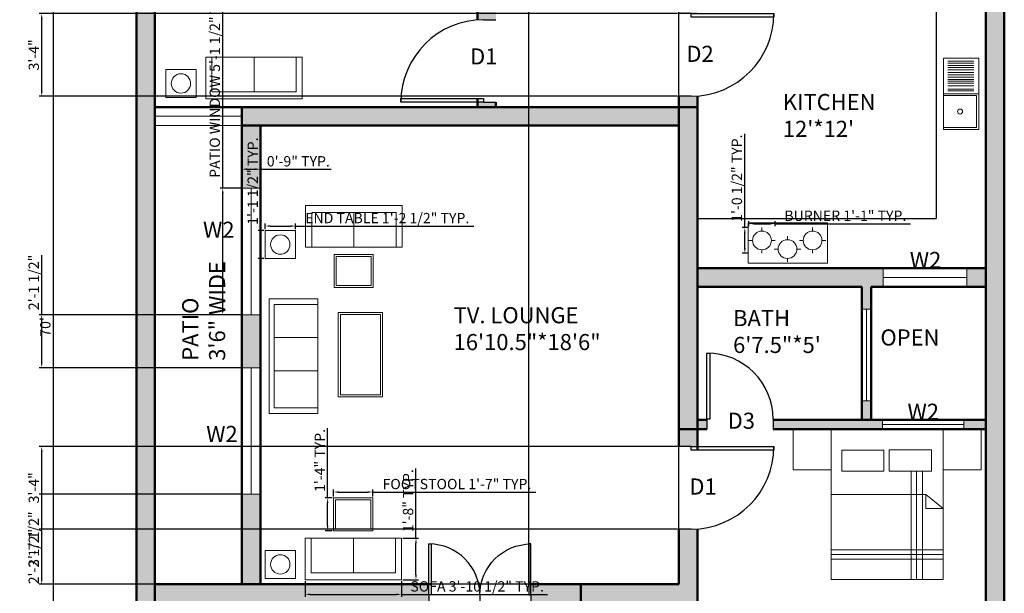
# Model space of a CAD drawing. Units: inches. Extents: x 2191 to 2715, y 2502 to 3448.
# Tile 2 of 3: x 2191 to 2668, y 2843 to 3120. Entities that reach past the tile are written whole.
import ezdxf

# ---------------------------------------------------------------- set-up
doc = ezdxf.new("R2010")
doc.units = ezdxf.units.IN
for name, color, linetype, lineweight in [('A-ANNO-DIMS', 2, 'Continuous', 18), ('A-AREA-IDEN', 130, 'Continuous', 25), ('A-EQPM', 8, 'Continuous', 18), ('A-FLOR-CASE', 9, 'Continuous', 25), ('A-FLOR-FIXT', 8, 'Continuous', 18), ('A-WALL-PATT', 150, 'Continuous', 13), ('DOOR', 52, 'Continuous', 25), ('FUR', 140, 'Continuous', 18), ('TEXT', 130, 'Continuous', 18), ('WALL', 150, 'Continuous', 50), ('WIN', 210, 'Continuous', 18)]:
    doc.layers.add(name, color=color, linetype=linetype, lineweight=lineweight)
doc.styles.get("Standard").update_dxf_attribs({"font": 'arial.ttf'})
doc.dimstyles.new('ISO-25', dxfattribs={"dimtxt": 5, "dimasz": 2.5, "dimexe": 1.25, "dimexo": 0.625, "dimtad": 1, "dimdec": 0, "dimlunit": 4, "dimtxsty": 'Standard', "dimcen": 2.5, "dimadec": 0, "dimazin": 0, "dimtfac": 1, "dimtdec": 0, "dimtmove": 0, "dimatfit": 3, "dimfxl": 1, "dimarcsym": 0})

# ---------------------------------------------------------------- blocks, each defined once
blk = doc.blocks.new('*U2')
for p, q in [((0, 0), (0, -6)), ((40, 0), (40, -6))]:
    blk.add_line(p, q)
blk.add_lwpolyline([(0, 0), (0, 40), (1.75, 40), (1.75, 0)], close=True)
blk.add_arc((0, 0), 40, 0, 90)
blk = doc.blocks.new('*D9')
at = {"layer": 'A-ANNO-DIMS', "color": 0, "lineweight": -2, "transparency": 16777216}
for p, q in [((2247.34, 3391.65), (2206.49, 3391.65)), ((2207.74, 3389.15), (2207.74, 2554.15)), ((2247.34, 2551.65), (2206.49, 2551.65))]:
    blk.add_line(p, q, dxfattribs=at)
at = {"layer": 'A-ANNO-DIMS', "color": 0, "lineweight": 100, "transparency": 16777216}
for points in [[(2207.32, 3389.15), (2208.15, 3389.15), (2207.74, 3391.65)], [(2207.32, 2554.15), (2208.15, 2554.15), (2207.74, 2551.65)]]:
    blk.add_solid(points, dxfattribs=at)
at = {"layer": 'Defpoints', "color": 0, "lineweight": 100, "transparency": 16777216}
for p in [(2247.96, 3391.65), (2207.74, 2551.65), (2247.96, 2551.65)]:
    blk.add_point(p, dxfattribs=at)
at = {"layer": 'A-ANNO-DIMS', "color": 0, "transparency": 16777216, "insert": (2204.56, 2971.65), "char_height": 5, "attachment_point": 5, "rotation": 90}
blk.add_mtext("70'", dxfattribs=at)
blk = doc.blocks.new('SOFA-TWO-SEAT')
for p, q in [((3.01, 20.24), (0, 20.24)), ((0, 20.24), (0, 0)), ((23.39, 20.24), (23.39, 3.45)), ((43.77, 20.24), (46.65, 20.24)), ((46.65, 20.24), (46.65, 20.24)), ((46.65, 20.24), (46.65, 0)), ((0, 0), (46.65, 0))]:
    blk.add_line(p, q)
blk.add_lwpolyline([(43.77, 3.45), (3.01, 3.45), (3.01, 20.24), (43.77, 20.24)], close=True)
blk = doc.blocks.new('TABLE-END-ROUND-ON-SQUARE')
blk.add_lwpolyline([(14.61, 0), (0, 0), (0, 13.55), (14.61, 13.55)], close=True)
blk.add_circle((7.31, 6.78), 4.68)
blk = doc.blocks.new('FOOTSTOOL')
for points in [[(0, 0), (19.01, 0), (19.01, 15.94), (0, 15.94)], [(1, 1), (18.01, 1), (18.01, 14.94), (1, 14.94)]]:
    blk.add_lwpolyline(points, close=True)
blk = doc.blocks.new('WINDOW-PATIO')
blk.add_line((4.5, 0), (4.5, 61.3))
blk.add_lwpolyline([(0, 0), (9, 0), (9, 61.3), (0, 61.3)], close=True)
blk = doc.blocks.new('COOKTOP-BURNER')
for p, q in [((6.38, 10.75), (6.38, 12.4)), ((0, 6.2), (1.83, 6.2)), ((10.93, 6.2), (12.76, 6.2)), ((6.38, 0), (6.38, 1.65))]:
    blk.add_line(p, q)
blk.add_circle((6.38, 6.2), 4.55)
blk = doc.blocks.new('*D16')
at = {"layer": 'A-ANNO-DIMS', "color": 0, "lineweight": -2, "transparency": 16777216}
for p, q in [((2329.62, 2848.52), (2329.62, 2840.89)), ((2376.27, 2848.52), (2376.27, 2840.89)), ((2332.12, 2842.14), (2373.77, 2842.14)), ((2376.27, 2842.14), (2446.96, 2842.14))]:
    blk.add_line(p, q, dxfattribs=at)
at = {"layer": 'A-ANNO-DIMS', "color": 0, "lineweight": 100, "transparency": 16777216}
for points in [[(2332.12, 2842.56), (2332.12, 2841.73), (2329.62, 2842.14)], [(2373.77, 2842.56), (2373.77, 2841.73), (2376.27, 2842.14)]]:
    blk.add_solid(points, dxfattribs=at)
at = {"layer": 'Defpoints', "color": 0, "lineweight": 100, "transparency": 16777216}
for p in [(2329.62, 2849.14), (2376.27, 2849.14), (2376.27, 2842.14)]:
    blk.add_point(p, dxfattribs=at)
at = {"layer": 'A-ANNO-DIMS', "color": 0, "transparency": 16777216, "insert": (2412.87, 2845.36), "char_height": 5, "attachment_point": 5}
blk.add_mtext('SOFA 3\'-10 1/2" TYP.', dxfattribs=at)
blk = doc.blocks.new('*D17')
at = {"layer": 'A-ANNO-DIMS', "color": 0, "lineweight": -2, "transparency": 16777216}
for p, q in [((2383.26, 2869.38), (2383.26, 2903.14)), ((2376.89, 2869.38), (2384.51, 2869.38)), ((2383.26, 2851.64), (2383.26, 2866.88)), ((2376.89, 2849.14), (2384.51, 2849.14))]:
    blk.add_line(p, q, dxfattribs=at)
at = {"layer": 'A-ANNO-DIMS', "color": 0, "lineweight": 100, "transparency": 16777216}
for points in [[(2382.85, 2866.88), (2383.68, 2866.88), (2383.26, 2869.38)], [(2382.85, 2851.64), (2383.68, 2851.64), (2383.26, 2849.14)]]:
    blk.add_solid(points, dxfattribs=at)
at = {"layer": 'Defpoints', "color": 0, "lineweight": 100, "transparency": 16777216}
for p in [(2376.27, 2869.38), (2383.26, 2869.38), (2376.27, 2849.14)]:
    blk.add_point(p, dxfattribs=at)
at = {"layer": 'A-ANNO-DIMS', "color": 0, "transparency": 16777216, "insert": (2380.09, 2887.51), "char_height": 5, "attachment_point": 5, "rotation": 90}
blk.add_mtext('1\'-8" TYP.', dxfattribs=at)
blk = doc.blocks.new('*D18')
at = {"layer": 'A-ANNO-DIMS', "color": 0, "lineweight": -2, "transparency": 16777216}
for p, q in [((2310.31, 3018.95), (2310.31, 3021.77)), ((2324.92, 3018.95), (2324.92, 3021.77)), ((2312.81, 3020.52), (2322.42, 3020.52)), ((2324.92, 3020.52), (2411.29, 3020.52))]:
    blk.add_line(p, q, dxfattribs=at)
at = {"layer": 'A-ANNO-DIMS', "color": 0, "lineweight": 100, "transparency": 16777216}
for points in [[(2312.81, 3020.94), (2312.81, 3020.1), (2310.31, 3020.52)], [(2322.42, 3020.94), (2322.42, 3020.1), (2324.92, 3020.52)]]:
    blk.add_solid(points, dxfattribs=at)
at = {"layer": 'Defpoints', "color": 0, "lineweight": 100, "transparency": 16777216}
for p in [(2310.31, 3018.33), (2324.92, 3020.52), (2324.92, 3018.33)]:
    blk.add_point(p, dxfattribs=at)
at = {"layer": 'A-ANNO-DIMS', "color": 0, "transparency": 16777216, "insert": (2369.36, 3023.73), "char_height": 5, "attachment_point": 5}
blk.add_mtext('END TABLE 1\'-2 1/2" TYP.', dxfattribs=at)
blk = doc.blocks.new('*D19')
at = {"layer": 'A-ANNO-DIMS', "color": 0, "lineweight": -2, "transparency": 16777216}
for p, q in [((2308.12, 3018.33), (2308.12, 3063.73)), ((2309.69, 3018.33), (2306.87, 3018.33)), ((2308.12, 3007.28), (2308.12, 3015.83)), ((2309.69, 3004.78), (2306.87, 3004.78))]:
    blk.add_line(p, q, dxfattribs=at)
at = {"layer": 'A-ANNO-DIMS', "color": 0, "lineweight": 100, "transparency": 16777216}
for points in [[(2307.7, 3015.83), (2308.54, 3015.83), (2308.12, 3018.33)], [(2307.7, 3007.28), (2308.54, 3007.28), (2308.12, 3004.78)]]:
    blk.add_solid(points, dxfattribs=at)
at = {"layer": 'Defpoints', "color": 0, "lineweight": 100, "transparency": 16777216}
for p in [(2308.12, 3018.33), (2310.31, 3018.33), (2310.31, 3004.78)]:
    blk.add_point(p, dxfattribs=at)
at = {"layer": 'A-ANNO-DIMS', "color": 0, "transparency": 16777216, "insert": (2304.91, 3042.28), "char_height": 5, "attachment_point": 5, "rotation": 90}
blk.add_mtext('1\'-1 1/2" TYP.', dxfattribs=at)
blk = doc.blocks.new('*D22')
at = {"layer": 'A-ANNO-DIMS', "color": 0, "lineweight": -2, "transparency": 16777216}
for p, q in [((2544.31, 3020.38), (2544.31, 3022.92)), ((2546.81, 3021.67), (2554.58, 3021.67)), ((2557.08, 3020.38), (2557.08, 3022.92)), ((2557.08, 3021.67), (2622.52, 3021.67))]:
    blk.add_line(p, q, dxfattribs=at)
at = {"layer": 'A-ANNO-DIMS', "color": 0, "lineweight": 100, "transparency": 16777216}
for points in [[(2546.81, 3022.09), (2546.81, 3021.25), (2544.31, 3021.67)], [(2554.58, 3022.09), (2554.58, 3021.25), (2557.08, 3021.67)]]:
    blk.add_solid(points, dxfattribs=at)
at = {"layer": 'Defpoints', "color": 0, "lineweight": 100, "transparency": 16777216}
for p in [(2557.08, 3021.67), (2544.31, 3019.76), (2557.08, 3019.76)]:
    blk.add_point(p, dxfattribs=at)
at = {"layer": 'A-ANNO-DIMS', "color": 0, "transparency": 16777216, "insert": (2591.05, 3024.85), "char_height": 5, "attachment_point": 5}
blk.add_mtext('BURNER 1\'-1" TYP.', dxfattribs=at)
blk = doc.blocks.new('*D23')
at = {"layer": 'A-ANNO-DIMS', "color": 0, "lineweight": -2, "transparency": 16777216}
for p, q in [((2542.4, 3019.76), (2542.4, 3065.16)), ((2543.69, 3019.76), (2541.15, 3019.76)), ((2542.4, 3009.86), (2542.4, 3017.26)), ((2543.69, 3007.36), (2541.15, 3007.36))]:
    blk.add_line(p, q, dxfattribs=at)
at = {"layer": 'A-ANNO-DIMS', "color": 0, "lineweight": 100, "transparency": 16777216}
for points in [[(2541.98, 3017.26), (2542.82, 3017.26), (2542.4, 3019.76)], [(2541.98, 3009.86), (2542.82, 3009.86), (2542.4, 3007.36)]]:
    blk.add_solid(points, dxfattribs=at)
at = {"layer": 'Defpoints', "color": 0, "lineweight": 100, "transparency": 16777216}
for p in [(2542.4, 3019.76), (2544.31, 3019.76), (2544.31, 3007.36)]:
    blk.add_point(p, dxfattribs=at)
at = {"layer": 'A-ANNO-DIMS', "color": 0, "transparency": 16777216, "insert": (2539.19, 3043.71), "char_height": 5, "attachment_point": 5, "rotation": 90}
blk.add_mtext('1\'-0 1/2" TYP.', dxfattribs=at)
blk = doc.blocks.new('*D24')
at = {"layer": 'A-ANNO-DIMS', "color": 0, "lineweight": -2, "transparency": 16777216}
for p, q in [((2343.35, 2889.49), (2343.35, 2892.97)), ((2362.36, 2889.49), (2362.36, 2892.97)), ((2345.85, 2891.72), (2359.86, 2891.72)), ((2362.36, 2891.72), (2441.32, 2891.72))]:
    blk.add_line(p, q, dxfattribs=at)
at = {"layer": 'A-ANNO-DIMS', "color": 0, "lineweight": 100, "transparency": 16777216}
for points in [[(2345.85, 2892.14), (2345.85, 2891.3), (2343.35, 2891.72)], [(2359.86, 2892.14), (2359.86, 2891.3), (2362.36, 2891.72)]]:
    blk.add_solid(points, dxfattribs=at)
at = {"layer": 'Defpoints', "color": 0, "lineweight": 100, "transparency": 16777216}
for p in [(2343.35, 2888.87), (2362.36, 2891.72), (2362.36, 2888.87)]:
    blk.add_point(p, dxfattribs=at)
at = {"layer": 'A-ANNO-DIMS', "color": 0, "transparency": 16777216, "insert": (2403.09, 2894.93), "char_height": 5, "attachment_point": 5}
blk.add_mtext('FOOTSTOOL 1\'-7" TYP.', dxfattribs=at)
blk = doc.blocks.new('*D25')
at = {"layer": 'A-ANNO-DIMS', "color": 0, "lineweight": -2, "transparency": 16777216}
for p, q in [((2340.5, 2888.87), (2340.5, 2922.62)), ((2342.73, 2888.87), (2339.25, 2888.87)), ((2340.5, 2875.43), (2340.5, 2886.37)), ((2342.73, 2872.93), (2339.25, 2872.93))]:
    blk.add_line(p, q, dxfattribs=at)
at = {"layer": 'A-ANNO-DIMS', "color": 0, "lineweight": 100, "transparency": 16777216}
for points in [[(2340.09, 2886.37), (2340.92, 2886.37), (2340.5, 2888.87)], [(2340.09, 2875.43), (2340.92, 2875.43), (2340.5, 2872.93)]]:
    blk.add_solid(points, dxfattribs=at)
at = {"layer": 'Defpoints', "color": 0, "lineweight": 100, "transparency": 16777216}
for p in [(2340.5, 2888.87), (2343.35, 2888.87), (2343.35, 2872.93)]:
    blk.add_point(p, dxfattribs=at)
at = {"layer": 'A-ANNO-DIMS', "color": 0, "transparency": 16777216, "insert": (2337.37, 2907), "char_height": 5, "attachment_point": 5, "rotation": 90}
blk.add_mtext('1\'-4" TYP.', dxfattribs=at)
blk = doc.blocks.new('*D26')
at = {"layer": 'A-ANNO-DIMS', "color": 0, "lineweight": -2, "transparency": 16777216}
for p, q in [((2289.77, 3038.86), (2289.77, 3139.97)), ((2298.34, 3038.86), (2288.52, 3038.86)), ((2289.77, 2980.06), (2289.77, 3036.36)), ((2298.34, 2977.56), (2288.52, 2977.56))]:
    blk.add_line(p, q, dxfattribs=at)
at = {"layer": 'A-ANNO-DIMS', "color": 0, "lineweight": 100, "transparency": 16777216}
for points in [[(2289.35, 3036.36), (2290.19, 3036.36), (2289.77, 3038.86)], [(2289.35, 2980.06), (2290.19, 2980.06), (2289.77, 2977.56)]]:
    blk.add_solid(points, dxfattribs=at)
at = {"layer": 'Defpoints', "color": 0, "lineweight": 100, "transparency": 16777216}
for p in [(2289.77, 3038.86), (2298.96, 3038.86), (2298.96, 2977.56)]:
    blk.add_point(p, dxfattribs=at)
at = {"layer": 'A-ANNO-DIMS', "color": 0, "transparency": 16777216, "insert": (2286.56, 3090.67), "char_height": 5, "attachment_point": 5, "rotation": 90}
blk.add_mtext('PATIO WINDOW 5\'-1 1/2" TYP.', dxfattribs=at)
blk = doc.blocks.new('*D27')
at = {"layer": 'A-ANNO-DIMS', "color": 0, "lineweight": -2, "transparency": 16777216}
for p, q in [((2298.96, 3039.48), (2298.96, 3049.3)), ((2301.46, 3048.05), (2305.46, 3048.05)), ((2307.96, 3039.48), (2307.96, 3049.3)), ((2307.96, 3048.05), (2342.19, 3048.05))]:
    blk.add_line(p, q, dxfattribs=at)
at = {"layer": 'A-ANNO-DIMS', "color": 0, "lineweight": 100, "transparency": 16777216}
for points in [[(2301.46, 3048.47), (2301.46, 3047.63), (2298.96, 3048.05)], [(2305.46, 3048.47), (2305.46, 3047.63), (2307.96, 3048.05)]]:
    blk.add_solid(points, dxfattribs=at)
at = {"layer": 'Defpoints', "color": 0, "lineweight": 100, "transparency": 16777216}
for p in [(2307.96, 3048.05), (2298.96, 3038.86), (2307.96, 3038.86)]:
    blk.add_point(p, dxfattribs=at)
at = {"layer": 'A-ANNO-DIMS', "color": 0, "transparency": 16777216, "insert": (2326.33, 3051.23), "char_height": 5, "attachment_point": 5}
blk.add_mtext('0\'-9" TYP.', dxfattribs=at)
blk = doc.blocks.new('*D28')
at = {"layer": 'A-ANNO-DIMS', "color": 0, "lineweight": -2, "transparency": 16777216}
for p, q in [((2509.84, 3123.41), (2200.91, 3123.41)), ((2202.16, 3085.91), (2202.16, 3120.91)), ((2509.84, 3083.41), (2200.91, 3083.41))]:
    blk.add_line(p, q, dxfattribs=at)
at = {"layer": 'A-ANNO-DIMS', "color": 0, "lineweight": 100, "transparency": 16777216}
for points in [[(2201.75, 3120.91), (2202.58, 3120.91), (2202.16, 3123.41)], [(2201.75, 3085.91), (2202.58, 3085.91), (2202.16, 3083.41)]]:
    blk.add_solid(points, dxfattribs=at)
at = {"layer": 'Defpoints', "color": 0, "lineweight": 100, "transparency": 16777216}
for p in [(2202.16, 3123.41), (2510.46, 3123.41), (2510.46, 3083.41)]:
    blk.add_point(p, dxfattribs=at)
at = {"layer": 'A-ANNO-DIMS', "color": 0, "transparency": 16777216, "insert": (2198.98, 3103.41), "char_height": 5, "attachment_point": 5, "rotation": 90}
blk.add_mtext('3\'-4"', dxfattribs=at)
blk = doc.blocks.new('*D31')
at = {"layer": 'A-ANNO-DIMS', "color": 0, "lineweight": -2, "transparency": 16777216}
for p, q in [((2509.84, 2913.75), (2200.91, 2913.75)), ((2202.16, 2876.25), (2202.16, 2911.25)), ((2509.84, 2873.75), (2200.91, 2873.75))]:
    blk.add_line(p, q, dxfattribs=at)
at = {"layer": 'A-ANNO-DIMS', "color": 0, "lineweight": 100, "transparency": 16777216}
for points in [[(2201.75, 2911.25), (2202.58, 2911.25), (2202.16, 2913.75)], [(2201.75, 2876.25), (2202.58, 2876.25), (2202.16, 2873.75)]]:
    blk.add_solid(points, dxfattribs=at)
at = {"layer": 'Defpoints', "color": 0, "lineweight": 100, "transparency": 16777216}
for p in [(2202.16, 2913.75), (2510.46, 2913.75), (2510.46, 2873.75)]:
    blk.add_point(p, dxfattribs=at)
at = {"layer": 'A-ANNO-DIMS', "color": 0, "transparency": 16777216, "insert": (2198.98, 2893.75), "char_height": 5, "attachment_point": 5, "rotation": 90}
blk.add_mtext('3\'-4"', dxfattribs=at)
blk = doc.blocks.new('*D32')
at = {"layer": 'A-ANNO-DIMS', "color": 0, "lineweight": -2, "transparency": 16777216}
for p, q in [((2509.84, 2873.75), (2200.91, 2873.75)), ((2202.16, 2849.65), (2202.16, 2871.25)), ((2509.84, 2847.15), (2200.91, 2847.15))]:
    blk.add_line(p, q, dxfattribs=at)
at = {"layer": 'A-ANNO-DIMS', "color": 0, "lineweight": 100, "transparency": 16777216}
for points in [[(2201.75, 2871.25), (2202.58, 2871.25), (2202.16, 2873.75)], [(2201.75, 2849.65), (2202.58, 2849.65), (2202.16, 2847.15)]]:
    blk.add_solid(points, dxfattribs=at)
at = {"layer": 'Defpoints', "color": 0, "lineweight": 100, "transparency": 16777216}
for p in [(2202.16, 2873.75), (2510.46, 2873.75), (2510.46, 2847.15)]:
    blk.add_point(p, dxfattribs=at)
at = {"layer": 'A-ANNO-DIMS', "color": 0, "transparency": 16777216, "insert": (2198.95, 2860.45), "char_height": 5, "attachment_point": 5, "rotation": 90}
blk.add_mtext('2\'-2 1/2"', dxfattribs=at)
blk = doc.blocks.new('*D33')
at = {"layer": 'A-ANNO-DIMS', "color": 0, "lineweight": -2, "transparency": 16777216}
for p, q in [((2437.84, 2847.78), (2437.84, 3438.7)), ((2440.34, 3437.45), (2507.96, 3437.45)), ((2510.46, 2847.78), (2510.46, 3438.7))]:
    blk.add_line(p, q, dxfattribs=at)
at = {"layer": 'A-ANNO-DIMS', "color": 0, "lineweight": 100, "transparency": 16777216}
for points in [[(2440.34, 3437.87), (2440.34, 3437.04), (2437.84, 3437.45)], [(2507.96, 3437.87), (2507.96, 3437.04), (2510.46, 3437.45)]]:
    blk.add_solid(points, dxfattribs=at)
at = {"layer": 'Defpoints', "color": 0, "lineweight": 100, "transparency": 16777216}
for p in [(2510.46, 3437.45), (2437.84, 2847.15), (2510.46, 2847.15)]:
    blk.add_point(p, dxfattribs=at)
at = {"layer": 'A-ANNO-DIMS', "color": 0, "transparency": 16777216, "insert": (2474.15, 3440.66), "char_height": 5, "attachment_point": 5}
blk.add_mtext('6\'-0 1/2"', dxfattribs=at)
blk = doc.blocks.new('*D34')
at = {"layer": 'A-ANNO-DIMS', "color": 0, "lineweight": -2, "transparency": 16777216}
for p, q in [((2298.34, 2890.63), (2200.91, 2890.63)), ((2202.16, 2849.65), (2202.16, 2888.13)), ((2298.34, 2847.15), (2200.91, 2847.15))]:
    blk.add_line(p, q, dxfattribs=at)
at = {"layer": 'A-ANNO-DIMS', "color": 0, "lineweight": 100, "transparency": 16777216}
for points in [[(2201.75, 2888.13), (2202.58, 2888.13), (2202.16, 2890.63)], [(2201.75, 2849.65), (2202.58, 2849.65), (2202.16, 2847.15)]]:
    blk.add_solid(points, dxfattribs=at)
at = {"layer": 'Defpoints', "color": 0, "lineweight": 100, "transparency": 16777216}
for p in [(2202.16, 2890.63), (2298.96, 2890.63), (2298.96, 2847.15)]:
    blk.add_point(p, dxfattribs=at)
at = {"layer": 'A-ANNO-DIMS', "color": 0, "transparency": 16777216, "insert": (2198.95, 2868.89), "char_height": 5, "attachment_point": 5, "rotation": 90}
blk.add_mtext('3\'-7 1/2"', dxfattribs=at)
blk = doc.blocks.new('*D35')
at = {"layer": 'A-ANNO-DIMS', "color": 0, "lineweight": -2, "transparency": 16777216}
for p, q in [((2202.16, 2977.56), (2202.16, 3006.34)), ((2298.34, 2977.56), (2200.91, 2977.56)), ((2202.16, 2954.43), (2202.16, 2975.06)), ((2298.34, 2951.93), (2200.91, 2951.93))]:
    blk.add_line(p, q, dxfattribs=at)
at = {"layer": 'A-ANNO-DIMS', "color": 0, "lineweight": 100, "transparency": 16777216}
for points in [[(2201.75, 2975.06), (2202.58, 2975.06), (2202.16, 2977.56)], [(2201.75, 2954.43), (2202.58, 2954.43), (2202.16, 2951.93)]]:
    blk.add_solid(points, dxfattribs=at)
at = {"layer": 'Defpoints', "color": 0, "lineweight": 100, "transparency": 16777216}
for p in [(2202.16, 2977.56), (2298.96, 2977.56), (2298.96, 2951.93)]:
    blk.add_point(p, dxfattribs=at)
at = {"layer": 'A-ANNO-DIMS', "color": 0, "transparency": 16777216, "insert": (2198.95, 2993.2), "char_height": 5, "attachment_point": 5, "rotation": 90}
blk.add_mtext('2\'-1 1/2"', dxfattribs=at)

msp = doc.modelspace()

# ---------------------------------------------------------------- hatches: boundary and pattern name
at = {"layer": 'A-WALL-PATT'}
h = msp.add_hatch(color=256, dxfattribs=at)
h.dxf.hatch_style = 1
h.paths.add_polyline_path([(2658.96, 3391.65), (2247.96, 3391.65), (2247.96, 3382.65), (2658.96, 3382.65)])
h.paths.add_polyline_path([(2256.96, 3382.65), (2247.96, 3382.65), (2247.96, 2561.19), (2256.96, 2561.19)])
h.paths.add_polyline_path([(2316.96, 3382.65), (2312.46, 3382.65), (2312.46, 3318.18), (2316.96, 3318.18)])
h.paths.add_polyline_path([(2412.96, 3279.15), (2308.33, 3279.15), (2308.33, 3270.15), (2412.96, 3270.15)])
h.paths.add_polyline_path([(2263, 3279.15), (2256.96, 3279.15), (2256.96, 3270.15), (2263, 3270.15)])
h.paths.add_polyline_path([(2421.96, 3323.7), (2412.96, 3323.7), (2412.96, 3279.15), (2421.96, 3279.15)])
h.paths.add_polyline_path([(2421.96, 3382.65), (2412.96, 3382.65), (2412.96, 3366.03), (2421.96, 3366.03)])
h.paths.add_polyline_path([(2421.96, 3279.15), (2412.96, 3279.15), (2412.96, 3270.15), (2412.96, 3120.46), (2421.96, 3120.46)])
h.paths.add_polyline_path([(2469.63, 3310.65), (2421.96, 3310.65), (2421.96, 3301.65), (2469.63, 3301.65)])
h.paths.add_polyline_path([(2594.46, 3310.65), (2549.09, 3310.65), (2549.09, 3301.65), (2594.46, 3301.65)])
h.paths.add_polyline_path([(2658.96, 3298.65), (2632.95, 3298.65), (2632.95, 3294.15), (2658.96, 3294.15)])
h.paths.add_polyline_path([(2600.93, 3298.65), (2598.96, 3298.65), (2598.96, 3328.67), (2594.46, 3328.67), (2594.46, 3310.65), (2594.46, 3294.15), (2594.46, 3284.36), (2598.96, 3284.36), (2598.96, 3294.15), (2600.93, 3294.15)])
h.paths.add_polyline_path([(2598.96, 3382.65), (2594.46, 3382.65), (2594.46, 3368.86), (2598.96, 3368.86), (2598.96, 3369.76)])
h.paths.add_polyline_path([(2667.96, 3391.65), (2658.96, 3391.65), (2658.96, 3382.65), (2658.96, 2551.65), (2667.96, 2551.65)])
h.paths.add_polyline_path([(2414.87, 2561.19), (2259.47, 2561.19), (2259.47, 2556.15), (2414.87, 2556.15)])
h.paths.add_polyline_path([(2259.47, 2561.19), (2247.96, 2561.19), (2247.96, 2551.65), (2259.47, 2551.65)])
h.paths.add_polyline_path([(2426.37, 2561.19), (2414.87, 2561.19), (2414.87, 2556.15), (2414.87, 2551.65), (2426.37, 2551.65), (2426.37, 2556.15)])
h.paths.add_polyline_path([(2667.96, 2556.15), (2426.37, 2556.15), (2426.37, 2551.65), (2667.96, 2551.65)])
h.paths.add_polyline_path([(2497.99, 2649.15), (2453.46, 2649.15), (2453.46, 2640.15), (2497.99, 2640.15)])
h.paths.add_polyline_path([(2462.96, 2693.64), (2453.46, 2693.64), (2453.46, 2649.15), (2462.96, 2649.15)])
h.paths.add_polyline_path([(2621.93, 2649.15), (2569.61, 2649.15), (2569.61, 2640.15), (2621.93, 2640.15)])
h.paths.add_polyline_path([(2610.96, 2721.15), (2606.46, 2721.15), (2606.46, 2649.15), (2610.96, 2649.15)])
h.paths.add_polyline_path([(2658.96, 2649.15), (2644.82, 2649.15), (2644.82, 2640.15), (2658.96, 2640.15)])
h.paths.add_polyline_path([(2462.96, 2784.15), (2453.46, 2784.15), (2453.46, 2733.49), (2459.46, 2733.49), (2462.96, 2733.49)])
h.paths.add_polyline_path([(2453.46, 2754.15), (2438.92, 2754.15), (2438.92, 2748.86), (2438.92, 2745.15), (2453.46, 2745.15)])
h.paths.add_polyline_path([(2389.52, 2754.15), (2256.96, 2754.15), (2256.96, 2745.15), (2389.52, 2745.15), (2389.52, 2748.86)])
h.paths.add_polyline_path([(2658.96, 2784.15), (2462.96, 2784.15), (2462.96, 2775.15), (2658.96, 2775.15)])
h.paths.add_polyline_path([(2658.96, 2725.65), (2639.65, 2725.65), (2639.65, 2721.68, -0.005), (2639.64, 2721.15), (2658.96, 2721.15)])
h.paths.add_polyline_path([(2613.17, 2725.65), (2606.46, 2725.65), (2606.46, 2721.15), (2610.96, 2721.15), (2613.17, 2721.15), (2613.17, 2721.68)])
h.paths.add_polyline_path([(2462.96, 2838.15), (2453.46, 2838.15), (2453.46, 2784.15), (2462.96, 2784.15)])
h.paths.add_polyline_path([(2389.52, 2847.15), (2256.96, 2847.15), (2256.96, 2838.15), (2389.52, 2838.15), (2389.52, 2841.86)])
h.paths.add_polyline_path([(2307.96, 2890.63), (2298.96, 2890.63), (2298.96, 2847.15), (2307.96, 2847.15)])
h.paths.add_polyline_path([(2462.96, 2847.15), (2453.96, 2847.15), (2438.92, 2847.15), (2438.92, 2841.86), (2438.92, 2838.15), (2453.96, 2838.15), (2462.96, 2838.15)])
h.paths.add_polyline_path([(2519.46, 2873.86, -0.01877), (2516.46, 2873.75), (2510.46, 2873.75), (2510.46, 2847.15), (2462.96, 2847.15), (2462.96, 2838.15), (2519.46, 2838.15)])
h.paths.add_polyline_path([(2519.46, 2922.15), (2510.46, 2922.15), (2510.46, 2913.75), (2516.46, 2913.75), (2519.46, 2913.75)])
h.paths.add_polyline_path([(2519.46, 2991.15), (2519.46, 3078.15), (2510.46, 3078.15), (2510.46, 3069.15), (2510.46, 2931.15), (2510.46, 2922.15), (2519.46, 2922.15), (2519.46, 2928.9), (2519.46, 2931.15)])
h.paths.add_polyline_path([(2609.08, 2926.65), (2556.08, 2926.65), (2556.08, 2922.15), (2609.08, 2922.15)])
h.paths.add_polyline_path([(2658.96, 2926.65), (2648.34, 2926.65), (2648.34, 2922.15), (2656.8, 2922.15), (2658.96, 2922.15)])
h.paths.add_polyline_path([(2603.46, 2931.15), (2603.46, 2935.9), (2598.96, 2935.9), (2598.96, 2931.15), (2598.96, 2926.65), (2603.46, 2926.65)])
h.paths.add_polyline_path([(2609.35, 3000.15), (2603.46, 3000.15), (2519.46, 3000.15), (2519.46, 2991.15), (2598.96, 2991.15), (2598.96, 2980.21), (2603.46, 2980.21), (2603.46, 2991.15), (2609.35, 2991.15)])
h.paths.add_polyline_path([(2658.96, 3000.15), (2649.75, 3000.15), (2649.75, 2991.15), (2658.96, 2991.15)])
h.paths.add_polyline_path([(2307.96, 2977.56), (2298.96, 2977.56), (2298.96, 2951.93), (2307.96, 2951.93)])
h.paths.add_polyline_path([(2307.96, 3069.15), (2298.96, 3069.15), (2298.96, 3038.86), (2307.96, 3038.86)])
h.paths.add_polyline_path([(2510.46, 3078.15), (2298.96, 3078.15), (2298.96, 3069.15), (2307.96, 3069.15), (2510.46, 3069.15)])
h.paths.add_polyline_path([(2421.96, 3080.46), (2415.96, 3080.46), (2412.96, 3080.46), (2412.96, 3078.15), (2421.96, 3078.15)])
h.paths.add_polyline_path([(2519.46, 3083.52, -0.01877), (2516.46, 3083.41), (2510.46, 3083.41), (2510.46, 3078.15), (2519.46, 3078.15)])
h.paths.add_polyline_path([(2519.46, 3127.65), (2510.46, 3127.65), (2510.46, 3123.41), (2516.46, 3123.41), (2519.46, 3123.41)])
h.paths.add_polyline_path([(2427.29, 3133.65), (2427.29, 3136.65), (2421.96, 3136.65), (2421.96, 3127.65), (2427.29, 3127.65)])
h.paths.add_polyline_path([(2598.96, 3136.65), (2467.29, 3136.65), (2467.29, 3127.65), (2598.96, 3127.65)])
h.paths.add_polyline_path([(2316.96, 3285.93), (2312.46, 3285.93), (2312.46, 3279.15), (2316.96, 3279.15)])
h.paths.add_polyline_path([(2658.96, 3234.15), (2598.96, 3234.15), (2598.96, 3229.65), (2658.96, 3229.65)])
h.paths.add_polyline_path([(2598.96, 3241.45), (2594.46, 3241.45), (2594.46, 3136.65), (2598.96, 3136.65)])
h.paths.add_polyline_path([(2658.96, 3136.65), (2632.67, 3136.65), (2632.67, 3127.65), (2658.96, 3127.65)])
h.paths.add_polyline_path([(2600.93, 3132.46), (2600.93, 3136.65), (2598.96, 3136.65), (2598.96, 3127.65), (2600.93, 3127.65)])
h.paths.add_polyline_path([(2524.07, 2926.65), (2519.46, 2926.65), (2519.46, 2922.15), (2524.07, 2922.15)])

# ---------------------------------------------------------------- linework, layer by layer
at = {"layer": 'A-EQPM'}
msp.add_lwpolyline([(2543.94, 3022.1), (2582.37, 3022.1), (2582.37, 3002.59), (2543.94, 3002.59)], close=True, dxfattribs=at)
at = {"layer": 'A-FLOR-CASE'}
for p, q in [((2634.96, 3127.65), (2634.96, 3024.15)), ((2519.46, 3000.15), (2519.46, 3024.15)), ((2519.46, 3024.15), (2634.96, 3024.15))]:
    msp.add_line(p, q, dxfattribs=at)
at = {"layer": 'A-FLOR-FIXT'}
for p, q in [((2640.66, 3100.35), (2653.22, 3100.35)), ((2640.66, 3099.44), (2653.22, 3099.44)), ((2640.66, 3098.33), (2653.22, 3098.33)), ((2640.66, 3097.22), (2653.22, 3097.22)), ((2640.66, 3096.11), (2653.22, 3096.11)), ((2640.66, 3094.9), (2653.22, 3094.9)), ((2640.66, 3093.74), (2653.22, 3093.74)), ((2640.66, 3092.68), (2653.22, 3092.68)), ((2640.66, 3091.47), (2653.22, 3091.47)), ((2640.66, 3090.72), (2653.22, 3090.72)), ((2640.66, 3089.76), (2653.22, 3089.76)), ((2640.66, 3088.35), (2653.22, 3088.35)), ((2638.54, 3084.5), (2655.63, 3084.5)), ((2639.42, 3084.5), (2651.98, 3084.5)), ((2640.66, 3086.83), (2653.22, 3086.83)), ((2640.66, 3085.93), (2653.22, 3085.93)), ((2640.66, 3084.5), (2653.22, 3084.5)), ((2640.66, 3084.5), (2653.22, 3084.5))]:
    msp.add_line(p, q, dxfattribs=at)
for points in [[(2638.54, 3101.76), (2655.63, 3101.76), (2655.63, 3067.23), (2638.54, 3067.23)], [(2654.55, 3068.23), (2638.54, 3068.23), (2638.54, 3083.72), (2654.55, 3083.72)]]:
    msp.add_lwpolyline(points, close=True, dxfattribs=at)
msp.add_circle((2646.54, 3075.97), 1.21, dxfattribs=at)
at = {"layer": 'FUR'}
for p, q in [((2335.85, 2985.26), (2312.27, 2985.26)), ((2312.27, 2985.26), (2312.27, 2929.67)), ((2335.85, 2982.56), (2335.85, 2985.26)), ((2314.7, 2966.5), (2335.85, 2966.5)), ((2314.7, 2950.42), (2335.85, 2950.42)), ((2332.61, 2950.42), (2335.85, 2950.42)), ((2335.85, 2929.67), (2335.85, 2934.08)), ((2312.27, 2929.67), (2335.85, 2929.67)), ((2622.92, 2901.85), (2622.92, 2849.27)), ((2625.49, 2901.85), (2625.49, 2849.27)), ((2628.3, 2901.85), (2628.3, 2849.27)), ((2584.13, 2890.54), (2629.92, 2890.54)), ((2629.92, 2890.54), (2629.92, 2883.72)), ((2638.42, 2883.72), (2629.92, 2890.54)), ((2629.92, 2883.72), (2638.42, 2883.72)), ((2638.42, 2863.71), (2584.13, 2863.71)), ((2638.42, 2861.49), (2584.13, 2861.49)), ((2638.42, 2859.27), (2584.13, 2859.27))]:
    msp.add_line(p, q, dxfattribs=at)
for points in [[(2335.85, 2982.56), (2314.7, 2982.56), (2314.7, 2932.51), (2335.85, 2932.51)], [(2345.66, 2937.74), (2367.05, 2937.74), (2367.05, 2978.66), (2345.66, 2978.66)], [(2346.66, 2938.74), (2366.05, 2938.74), (2366.05, 2977.66), (2346.66, 2977.66)], [(2565.75, 2922.15), (2584.13, 2922.15), (2584.13, 2902.4), (2565.75, 2902.4)], [(2589.3, 2912.06), (2609.73, 2912.06), (2609.73, 2901.76), (2589.3, 2901.76)], [(2612.26, 2912.14), (2632.69, 2912.14), (2632.69, 2901.85), (2612.26, 2901.85)]]:
    msp.add_lwpolyline(points, close=True, dxfattribs=at)
for points in [[(2638.42, 2922.15), (2638.42, 2849.27), (2584.13, 2849.27), (2584.13, 2922.15), (2609.08, 2922.15)], [(2648.34, 2922.15), (2656.8, 2922.15), (2656.8, 2902.4), (2638.42, 2902.4), (2638.42, 2922.15)]]:
    msp.add_lwpolyline(points, dxfattribs=at)
at = {"layer": 'WALL'}
for p, q in [((2247.96, 2551.65), (2247.96, 3391.65)), ((2667.96, 3391.65), (2667.96, 2551.65)), ((2256.96, 2561.19), (2256.96, 3382.65)), ((2658.96, 3382.65), (2658.96, 2551.65)), ((2412.96, 3120.35), (2412.96, 3270.15)), ((2510.46, 3069.15), (2510.46, 3083.41)), ((2519.46, 3078.15), (2519.46, 3083.52)), ((2256.96, 3078.15), (2412.96, 3078.15)), ((2298.96, 2847.15), (2298.96, 3078.15)), ((2298.96, 3078.15), (2519.46, 3078.15)), ((2412.96, 3078.15), (2412.96, 3082.21)), ((2421.96, 3078.15), (2421.96, 3080.46)), ((2519.46, 3078.15), (2519.46, 2931.15)), ((2307.96, 3069.15), (2298.96, 3069.15)), ((2307.96, 2847.15), (2307.96, 3069.15)), ((2307.96, 2847.15), (2307.96, 3069.15)), ((2307.96, 3069.15), (2510.46, 3069.15)), ((2510.46, 3069.15), (2510.46, 2931.15)), ((2519.46, 3000.15), (2603.46, 3000.15)), ((2603.46, 3000.15), (2658.96, 3000.15)), ((2519.46, 2931.15), (2519.46, 2991.15)), ((2519.46, 2991.15), (2598.96, 2991.15)), ((2598.96, 2991.15), (2598.96, 2931.15)), ((2603.46, 2991.15), (2603.46, 2931.15)), ((2603.46, 2991.15), (2658.96, 2991.15)), ((2510.46, 2922.15), (2510.46, 2931.15)), ((2519.46, 2931.15), (2519.46, 2926.65)), ((2598.96, 2931.15), (2598.96, 2926.65)), ((2603.46, 2931.15), (2603.46, 2926.65)), ((2519.46, 2928.9), (2519.46, 2912)), ((2519.46, 2926.65), (2524.07, 2926.65)), ((2556.08, 2926.65), (2658.96, 2926.65)), ((2519.46, 2922.15), (2510.46, 2922.15)), ((2510.46, 2922.15), (2510.46, 2913.75)), ((2519.46, 2922.15), (2524.07, 2922.15)), ((2556.08, 2922.15), (2658.96, 2922.15)), ((2654.96, 2922.15), (2658.96, 2922.15)), ((2658.96, 2784.15), (2658.96, 2922.15)), ((2510.46, 2873.75), (2510.46, 2847.15)), ((2519.46, 2873.86), (2519.46, 2838.15)), ((2256.96, 2847.15), (2390.6, 2847.15)), ((2256.96, 2847.15), (2298.96, 2847.15)), ((2437.84, 2847.15), (2453.96, 2847.15)), ((2462.96, 2847.15), (2453.96, 2847.15)), ((2462.96, 2784.15), (2462.96, 2847.15)), ((2510.46, 2847.15), (2462.96, 2847.15))]:
    msp.add_line(p, q, dxfattribs=at)
for points in [[(2658.96, 3391.65), (2667.96, 3391.65), (2667.96, 2551.65), (2658.96, 2551.65)], [(2247.96, 2561.19), (2256.96, 2561.19), (2256.96, 3382.65), (2247.96, 3382.65)]]:
    msp.add_lwpolyline(points, close=True, dxfattribs=at)
at = {"layer": 'WIN'}
for p, q in [((2298.96, 3078.15), (2256.96, 3078.15)), ((2256.96, 3069.15), (2256.96, 3078.15)), ((2256.96, 3078.15), (2298.96, 3078.15)), ((2298.96, 3078.15), (2256.96, 3078.15)), ((2298.96, 3069.15), (2298.96, 3078.15)), ((2256.96, 3073.65), (2298.96, 3073.65)), ((2298.96, 3069.15), (2256.96, 3069.15)), ((2609.35, 2995.65), (2649.75, 2995.65)), ((2601.21, 2935.9), (2601.21, 2980.21)), ((2609.08, 2924.4), (2648.34, 2924.4))]:
    msp.add_line(p, q, dxfattribs=at)
for points in [[(2609.35, 2991.15), (2649.75, 2991.15), (2649.75, 3000.15), (2609.35, 3000.15)], [(2598.96, 2980.21), (2603.46, 2980.21), (2603.46, 2935.9), (2598.96, 2935.9)], [(2609.08, 2922.15), (2648.34, 2922.15), (2648.34, 2926.65), (2609.08, 2926.65)]]:
    msp.add_lwpolyline(points, close=True, dxfattribs=at)

# ---------------------------------------------------------------- block references
at = {"layer": 'A-EQPM'}
for p in [(2544.32, 3007.36), (2568.81, 3007.36), (2556.66, 3003.17)]:
    msp.add_blockref('COOKTOP-BURNER', p, dxfattribs=at)
at = {"layer": 'DOOR'}
for p, rotation in [((2516.46, 3123.41), 270), ((2415.96, 3080.46), 90), ((2516.46, 2913.75), 270)]:
    msp.add_blockref('*U2', p, dxfattribs=dict(at, rotation=rotation))
for p, xscale, yscale, zscale in [((2524.07, 2926.96), 0.8003192358726801, 0.8003192358726801, 0.8003192358726801), ((2389.52, 2841.86), 0.617424543084726, 0.617424543084726, 0.617424543084726), ((2438.92, 2841.86), -0.617424543084726, 0.617424543084726, 0.617424543084726)]:
    msp.add_blockref('*U2', p, dxfattribs=dict(at, xscale=xscale, yscale=yscale, zscale=zscale))
at = {"layer": 'FUR'}
for name, p in [('SOFA-TWO-SEAT', (2281.51, 3082.05)), ('TABLE-END-ROUND-ON-SQUARE', (2262.21, 3082.79)), ('TABLE-END-ROUND-ON-SQUARE', (2310.31, 3004.78)), ('FOOTSTOOL', (2343.35, 2872.93)), ('SOFA-TWO-SEAT', (2329.61, 2849.14)), ('TABLE-END-ROUND-ON-SQUARE', (2310.31, 2849.88))]:
    msp.add_blockref(name, p, dxfattribs=at)
at = {"layer": 'FUR', "extrusion": (0, 0, -1), "zscale": -1, "rotation": 180}
for name, p in [('SOFA-TWO-SEAT', (-2329.86, 3030.49)), ('FOOTSTOOL', (-2343.6, 3006.71))]:
    msp.add_blockref(name, p, dxfattribs=at)
at = {"layer": 'WIN'}
for p in [(2298.96, 2977.56), (2298.96, 2890.63)]:
    msp.add_blockref('WINDOW-PATIO', p, dxfattribs=at)

# ---------------------------------------------------------------- texts
at = {"layer": 'A-AREA-IDEN', "attachment_point": 1}
for s, insert, char_height in [("KITCHEN\\P12'*12'", (2560.81, 3084.48), 7.795), ('TV. LOUNGE\\P16\'10.5"*18\'6"', (2401.48, 2981.22), 7.7945), ('BATH\\P6\'7.5"*5\'', (2536.71, 2979.84), 7.795), ('OPEN', (2608.01, 2970.46), 7.795)]:
    msp.add_mtext_dynamic_manual_height_columns(s, width=100.7314, gutter_width=38.97, heights=[0], dxfattribs=dict(at, insert=insert, char_height=char_height))
at = {"layer": 'A-AREA-IDEN', "insert": (2270.14, 2955.28), "char_height": 7.795, "attachment_point": 1, "rotation": 90}
msp.add_mtext_dynamic_manual_height_columns('PATIO\\P3\'6" WIDE', width=100.7314, gutter_width=38.97, heights=[0], dxfattribs=at)
at = {"layer": 'TEXT', "char_height": 7.795, "attachment_point": 1}
for s, insert in [('D2', (2514.12, 3107.81)), ('D1', (2409.46, 3106.55)), ('W2', (2280.21, 3022.61)), ('W2', (2622.23, 3007.98)), ('W2', (2621.13, 2934.48)), ('D3', (2534.09, 2930.12)), ('W2', (2281.75, 2923.73)), ('D1', (2515.56, 2898.28))]:
    msp.add_mtext_dynamic_manual_height_columns(s, width=100.7314, gutter_width=38.97, heights=[0], dxfattribs=dict(at, insert=insert))

# ---------------------------------------------------------------- dimensions: what is measured, and where the dimension line sits
at = {"layer": 'A-ANNO-DIMS'}
dim = msp.add_linear_dim(base=(2510.46, 3437.45), p1=(2437.84, 2847.15), p2=(2510.46, 2847.15), dimstyle='ISO-25', override={"dimdec": 1, "dimlfac": 1, "dimrnd": 0, "dimzin": 1, "dimdsep": 46, "dimlunit": 4, "dimfrac": 2}, dxfattribs=at)
dim.commit()
dim.dimension.update_dxf_attribs({"geometry": '*D33', "text_midpoint": (2474.15, 3440.66)})
for base, p1, p2, override, picture, middle in [((2207.74, 2551.65), (2247.96, 3391.65), (2247.96, 2551.65), {"dimclrd": 0, "dimclre": 0, "dimclrt": 0}, '*D9', (2204.56, 2971.65)), ((2202.16, 3123.41), (2510.46, 3083.41), (2510.46, 3123.41), {"dimdec": 1, "dimlfac": 1, "dimrnd": 0, "dimzin": 1, "dimdsep": 46, "dimlunit": 4, "dimfrac": 2}, '*D28', (2198.98, 3103.41)), ((2202.16, 2977.56), (2298.96, 2951.93), (2298.96, 2977.56), {"dimdec": 1, "dimlfac": 1, "dimrnd": 0, "dimzin": 1, "dimdsep": 46, "dimlunit": 4, "dimfrac": 2}, '*D35', (2198.95, 2993.2)), ((2202.16, 2913.75), (2510.46, 2873.75), (2510.46, 2913.75), {"dimdec": 1, "dimlfac": 1, "dimrnd": 0, "dimzin": 1, "dimdsep": 46, "dimlunit": 4, "dimfrac": 2}, '*D31', (2198.98, 2893.75)), ((2202.16, 2890.63), (2298.96, 2847.15), (2298.96, 2890.63), {"dimdec": 1, "dimlfac": 1, "dimrnd": 0, "dimzin": 1, "dimdsep": 46, "dimlunit": 4, "dimfrac": 2}, '*D34', (2198.95, 2868.89)), ((2202.16, 2873.75), (2510.46, 2847.15), (2510.46, 2873.75), {"dimdec": 1, "dimlfac": 1, "dimrnd": 0, "dimzin": 1, "dimdsep": 46, "dimlunit": 4, "dimfrac": 2}, '*D32', (2198.95, 2860.45))]:
    dim = msp.add_linear_dim(base=base, p1=p1, p2=p2, angle=90, dimstyle='ISO-25', override=override, dxfattribs=at)
    dim.commit()
    dim.dimension.update_dxf_attribs({"geometry": picture, "text_midpoint": middle})
for base, p1, p2, text, picture, middle in [((2289.77, 3038.86), (2298.96, 2977.56), (2298.96, 3038.86), 'PATIO WINDOW <> TYP.', '*D26', (2286.56, 3090.67)), ((2308.1186, 3018.327), (2310.3103, 3004.7754), (2310.3103, 3018.327), '<> TYP.', '*D19', (2304.9083, 3042.2808)), ((2542.4, 3019.76), (2544.31, 3007.36), (2544.31, 3019.76), '<> TYP.', '*D23', (2539.19, 3043.71)), ((2340.5, 2888.87), (2343.35, 2872.93), (2343.35, 2888.87), '<> TYP.', '*D25', (2337.37, 2907)), ((2383.26, 2869.38), (2376.27, 2849.14), (2376.27, 2869.38), '<> TYP.', '*D17', (2380.09, 2887.51))]:
    dim = msp.add_linear_dim(base=base, p1=p1, p2=p2, angle=90, text=text, dimstyle='ISO-25', override={"dimdec": 1, "dimlfac": 1, "dimrnd": 0, "dimzin": 1, "dimdsep": 46, "dimlunit": 4, "dimfrac": 2}, dxfattribs=at)
    dim.commit()
    dim.dimension.update_dxf_attribs({"geometry": picture, "text_midpoint": middle})
for base, p1, p2, text, picture, middle in [((2307.96, 3048.05), (2298.96, 3038.86), (2307.96, 3038.86), '<> TYP.', '*D27', (2326.33, 3051.23)), ((2324.92, 3020.52), (2310.31, 3018.33), (2324.92, 3018.33), 'END TABLE <> TYP.', '*D18', (2369.36, 3023.73)), ((2557.08, 3021.67), (2544.31, 3019.76), (2557.08, 3019.76), 'BURNER <> TYP.', '*D22', (2591.05, 3024.85)), ((2362.36, 2891.72), (2343.35, 2888.87), (2362.36, 2888.87), 'FOOTSTOOL <> TYP.', '*D24', (2403.09, 2894.93)), ((2376.2667, 2842.1443), (2329.6151, 2849.1421), (2376.2667, 2849.1421), 'SOFA <> TYP.', '*D16', (2412.8655, 2845.358))]:
    dim = msp.add_linear_dim(base=base, p1=p1, p2=p2, text=text, dimstyle='ISO-25', override={"dimdec": 1, "dimlfac": 1, "dimrnd": 0, "dimzin": 1, "dimdsep": 46, "dimlunit": 4, "dimfrac": 2}, dxfattribs=at)
    dim.commit()
    dim.dimension.update_dxf_attribs({"geometry": picture, "text_midpoint": middle})

doc.saveas('drawing.dxf')
